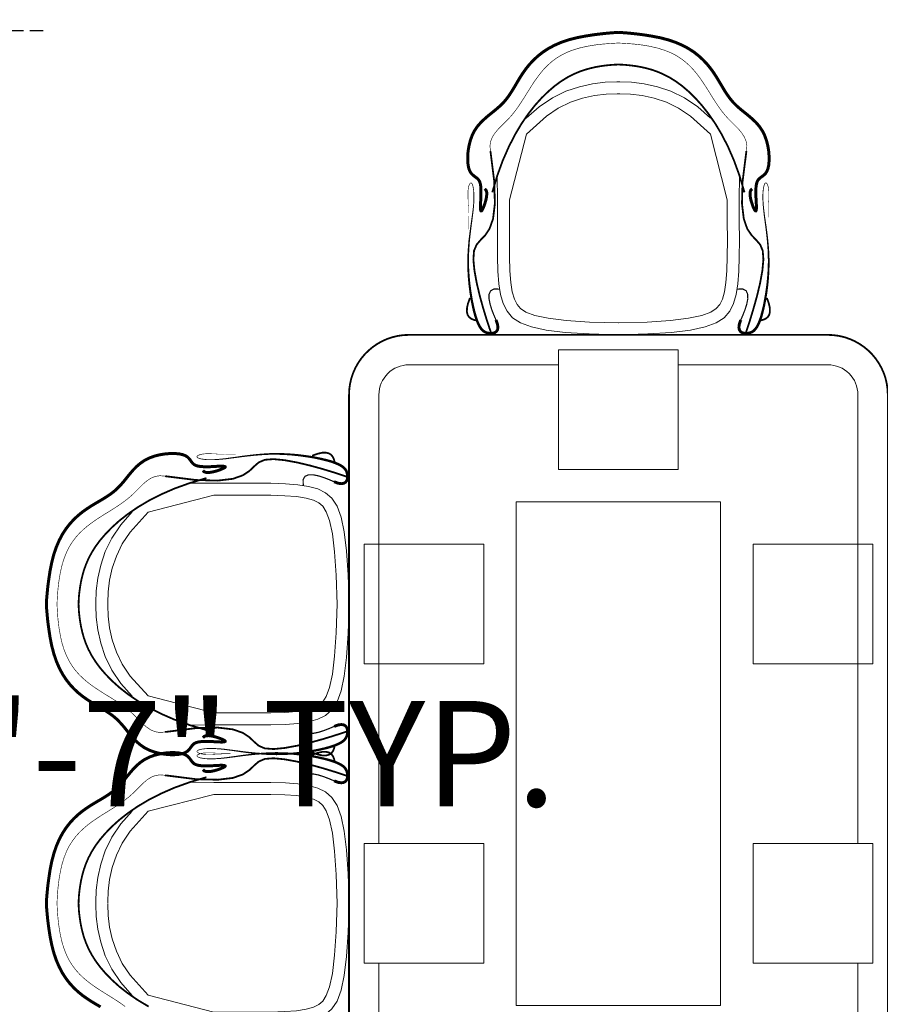
# Model space of a CAD drawing. Units: inches. Extents: x 513 to 1142, y 396 to 927.
# Tile 17 of 31: x 786 to 818, y 728 to 766. Entities that reach past the tile are written whole.
import ezdxf

# ---------------------------------------------------------------- set-up
doc = ezdxf.new("R2010")
doc.units = ezdxf.units.IN
doc.header["$MEASUREMENT"] = 0
doc.linetypes.add('DASHED', pattern=[0.75, 0.5, -0.25])
doc.layers.add('A-ANNO-DIMS', color=2, linetype='DASHED', lineweight=18)
doc.layers.add('furniture', color=92, linetype='Continuous', lineweight=18)
doc.styles.get("Standard").update_dxf_attribs({"font": 'arial.ttf'})
doc.dimstyles.get("Standard").update_dxf_attribs({"dimtxt": 4, "dimasz": 0.18, "dimexe": 0.18, "dimexo": 0.0625, "dimgap": 0.09, "dimtad": 0, "dimtih": 1, "dimtoh": 1, "dimdec": 0, "dimrnd": 6, "dimzin": 0, "dimdsep": 46, "dimlunit": 3, "dimtxsty": 'Standard', "dimcen": 0.09, "dimadec": 0, "dimazin": 0, "dimtfac": 1, "dimtdec": 0, "dimtofl": 0, "dimtmove": 0, "dimatfit": 3, "dimfxl": 1, "dimtolj": 1, "dimtzin": 0, "dimarcsym": 0})

# ---------------------------------------------------------------- blocks, each defined once
blk = doc.blocks.new('ОГ55_на6персон_стол1400х900')
for points, const_width in [([(-423.2, 694.5), (-418.9, 701.9), (-414.4, 709.4), (-409.5, 716.9), (-404.2, 724.4), (-398.3, 731.7), (-391.7, 738.8), (-384.3, 745.6), (-376.1, 752), (-366.9, 758), (-356.7, 763.4), (-345.4, 768.3), (-333, 772.5), (-319.5, 776), (-305.4, 778.8), (-291.5, 780.9), (-278.6, 782.6), (-267.2, 783.7), (-258.2, 784.5), (-252.2, 784.9), (-250, 785)], 5), ([(-26.6, 523.4), (-28.8, 521.4), (-29.9, 518.2), (-30.1, 514.2), (-29.6, 509.6), (-28.6, 504.8), (-27.3, 500.1), (-25.8, 495.7), (-24.3, 492), (-23, 489.2), (-22, 487.3), (-21.1, 486.4), (-20.4, 486.4), (-19.9, 487.3), (-19.6, 489.1), (-19.4, 491.8), (-19.5, 495.4), (-19.7, 499.8), (-20, 504.9), (-20.3, 510.3), (-20.4, 516), (-20.4, 521.5), (-20.1, 526.8), (-19.4, 531.5), (-18.2, 535.5), (-16.5, 538.5), (-14.3, 540.8), (-11.8, 542.8), (-9.2, 544.6), (-6.6, 546.7), (-4.1, 549.3), (-1.9, 552.7), (-0.2, 557.2), (1.1, 563.1), (1.7, 570.2), (1.7, 578.1), (1, 586.6), (-0.4, 595.4), (-2.6, 604.2), (-5.7, 612.7), (-9.6, 620.6), (-14.5, 627.7), (-20, 634.2), (-26.1, 640.1), (-32.5, 645.6), (-39.1, 650.9), (-45.7, 656.2), (-51.9, 661.7), (-57.8, 667.5), (-63.1, 673.7), (-67.9, 680.3), (-72.4, 687.3), (-76.8, 694.5), (-81.1, 701.9), (-85.6, 709.4), (-90.5, 716.9), (-95.8, 724.4), (-101.7, 731.7), (-108.3, 738.8), (-115.7, 745.6), (-123.9, 752), (-133.1, 758), (-143.3, 763.4), (-154.6, 768.3), (-167, 772.5), (-180.5, 776), (-194.6, 778.8), (-208.5, 780.9), (-221.4, 782.6), (-232.8, 783.7), (-241.8, 784.5), (-247.8, 784.9), (-250, 785)], 5), ([(26.6, 523.4), (28.8, 521.4), (29.9, 518.2), (30.1, 514.2), (29.6, 509.6), (28.6, 504.8), (27.3, 500.1), (25.8, 495.7), (24.3, 492), (23, 489.2), (22, 487.3), (21.1, 486.4), (20.4, 486.4), (19.9, 487.3), (19.6, 489.1), (19.4, 491.8), (19.5, 495.4), (19.7, 499.8), (20, 504.9), (20.3, 510.3), (20.4, 516), (20.4, 521.5), (20.1, 526.8), (19.4, 531.5), (18.2, 535.5), (16.5, 538.5), (14.3, 540.8), (11.8, 542.8), (9.2, 544.6), (6.6, 546.7), (4.1, 549.3), (1.9, 552.7), (0.2, 557.2), (-1.1, 563.1), (-1.7, 570.2), (-1.7, 578.1), (-1, 586.6), (0.4, 595.4), (2.6, 604.2), (5.7, 612.7), (9.6, 620.6), (14.5, 627.7), (20, 634.2), (26.1, 640.1), (32.5, 645.6), (39.1, 650.9), (45.7, 656.2), (51.9, 661.7), (57.8, 667.5), (63.1, 673.7), (67.9, 680.3), (72.4, 687.3), (76.8, 694.5), (81.1, 701.9), (85.6, 709.4), (90.5, 716.9), (95.8, 724.4), (101.7, 731.7), (108.3, 738.8), (115.7, 745.6), (123.9, 752), (133.1, 758), (143.3, 763.4), (154.6, 768.3), (167, 772.5), (180.5, 776), (194.6, 778.8), (208.5, 780.9), (221.4, 782.6), (232.8, 783.7), (241.8, 784.5), (247.8, 784.9), (250, 785)], 5), ([(473.4, 523.4), (471.2, 521.4), (470.1, 518.2), (469.9, 514.2), (470.4, 509.6), (471.4, 504.8), (472.7, 500.1), (474.2, 495.7), (475.7, 492), (477, 489.2), (478, 487.3), (478.9, 486.4), (479.6, 486.4), (480.1, 487.3), (480.4, 489.1), (480.6, 491.8), (480.5, 495.4), (480.3, 499.8), (480, 504.9), (479.7, 510.3), (479.6, 516), (479.6, 521.5), (479.9, 526.8), (480.6, 531.5), (481.8, 535.5), (483.5, 538.5), (485.7, 540.8), (488.2, 542.8), (490.8, 544.6), (493.4, 546.7), (495.9, 549.3), (498.1, 552.7), (499.8, 557.2), (501.1, 563.1), (501.7, 570.2), (501.7, 578.1), (501, 586.6), (499.6, 595.4), (497.4, 604.2), (494.3, 612.7), (490.4, 620.6), (485.5, 627.7), (480, 634.2), (473.9, 640.1), (467.5, 645.6), (460.9, 650.9), (454.3, 656.2), (448.1, 661.7), (442.2, 667.5), (436.9, 673.7), (432.1, 680.3), (427.6, 687.3), (423.2, 694.5), (418.9, 701.9), (414.4, 709.4), (409.5, 716.9), (404.2, 724.4), (398.3, 731.7), (391.7, 738.8), (384.3, 745.6), (376.1, 752), (366.9, 758), (356.7, 763.4), (345.4, 768.3), (333, 772.5), (319.5, 776), (305.4, 778.8), (291.5, 780.9), (278.6, 782.6), (267.2, 783.7), (258.2, 784.5), (252.2, 784.9), (250, 785)], 5), ([(-422.8, 653.3), (-417.9, 659.9), (-413.3, 666.7), (-408.8, 673.7), (-404.4, 680.7), (-400, 687.9), (-395.5, 695), (-390.8, 702.2), (-385.8, 709.3), (-380.5, 716.3), (-374.7, 723.1), (-368.5, 729.6), (-361.7, 735.7), (-354.1, 741.4), (-345.9, 746.6), (-336.7, 751.2), (-326.7, 755.2), (-315.5, 758.7), (-303.3, 761.5), (-289.8, 763.8), (-274.9, 765.6), (-258.6, 766.8), (-250, 767.1)], 1), ([(-36.2, 586.5), (-35.4, 595.2), (-36.6, 603), (-39.5, 610.1), (-43.7, 616.6), (-48.9, 622.8), (-54.7, 628.7), (-60.7, 634.6), (-66.6, 640.6), (-72.1, 646.8), (-77.2, 653.3), (-82.1, 659.9), (-86.7, 666.7), (-91.2, 673.7), (-95.6, 680.7), (-100, 687.9), (-104.5, 695), (-109.2, 702.2), (-114.2, 709.3), (-119.5, 716.3), (-125.3, 723.1), (-131.5, 729.6), (-138.3, 735.7), (-145.9, 741.4), (-154.1, 746.6), (-163.3, 751.2), (-173.3, 755.2), (-184.5, 758.7), (-196.7, 761.5), (-210.2, 763.8), (-225.1, 765.6), (-241.4, 766.8), (-250, 767.1)], 1), ([(36.2, 586.5), (35.4, 595.2), (36.6, 603), (39.5, 610.1), (43.7, 616.6), (48.9, 622.8), (54.7, 628.7), (60.7, 634.6), (66.6, 640.6), (72.1, 646.8), (77.2, 653.3), (82.1, 659.9), (86.7, 666.7), (91.2, 673.7), (95.6, 680.7), (100, 687.9), (104.5, 695), (109.2, 702.2), (114.2, 709.3), (119.5, 716.3), (125.3, 723.1), (131.5, 729.6), (138.3, 735.7), (145.9, 741.4), (154.1, 746.6), (163.3, 751.2), (173.3, 755.2), (184.5, 758.7), (196.7, 761.5), (210.2, 763.8), (225.1, 765.6), (241.4, 766.8), (250, 767.1)], 1), ([(463.8, 586.5), (464.6, 595.2), (463.4, 603), (460.5, 610.1), (456.3, 616.6), (451.1, 622.8), (445.3, 628.7), (439.3, 634.6), (433.4, 640.6), (427.9, 646.8), (422.8, 653.3), (417.9, 659.9), (413.3, 666.7), (408.8, 673.7), (404.4, 680.7), (400, 687.9), (395.5, 695), (390.8, 702.2), (385.8, 709.3), (380.5, 716.3), (374.7, 723.1), (368.5, 729.6), (361.7, 735.7), (354.1, 741.4), (345.9, 746.6), (336.7, 751.2), (326.7, 755.2), (315.5, 758.7), (303.3, 761.5), (289.8, 763.8), (274.9, 765.6), (258.6, 766.8), (250, 767.1)], 1), ([(-422.7, 614.1), (-411.8, 632.4), (-400.6, 648.7), (-389.4, 663), (-378.2, 675.4), (-367.2, 686.1), (-356.5, 695.3), (-346, 703), (-335.8, 709.4), (-325.7, 714.7), (-315.9, 718.9), (-306.4, 722.3), (-297, 724.9), (-287.9, 727), (-279.3, 728.5), (-271.3, 729.6), (-264.3, 730.4), (-258.4, 730.8), (-253.9, 731), (-251, 731.1), (-250, 731.1)], 3), ([(-39.4, 517.6), (-47.7, 545.4), (-56.8, 570.7), (-66.8, 593.6), (-77.3, 614.1), (-88.2, 632.4), (-99.4, 648.7), (-110.6, 663), (-121.8, 675.4), (-132.8, 686.1), (-143.5, 695.3), (-154, 703), (-164.2, 709.4), (-174.3, 714.7), (-184.1, 718.9), (-193.6, 722.3), (-203, 724.9), (-212.1, 727), (-220.7, 728.5), (-228.7, 729.6), (-235.7, 730.4), (-241.6, 730.8), (-246.1, 731), (-249, 731.1), (-250, 731.1)], 3), ([(39.4, 517.6), (47.7, 545.4), (56.8, 570.7), (66.8, 593.6), (77.3, 614.1), (88.2, 632.4), (99.4, 648.7), (110.6, 663), (121.8, 675.4), (132.8, 686.1), (143.5, 695.3), (154, 703), (164.2, 709.4), (174.3, 714.7), (184.1, 718.9), (193.6, 722.3), (203, 724.9), (212.1, 727), (220.7, 728.5), (228.7, 729.6), (235.7, 730.4), (241.6, 730.8), (246.1, 731), (249, 731.1), (250, 731.1)], 3), ([(460.6, 517.6), (452.3, 545.4), (443.2, 570.7), (433.2, 593.6), (422.7, 614.1), (411.8, 632.4), (400.6, 648.7), (389.4, 663), (378.2, 675.4), (367.2, 686.1), (356.5, 695.3), (346, 703), (335.8, 709.4), (325.7, 714.7), (315.9, 718.9), (306.4, 722.3), (297, 724.9), (287.9, 727), (279.3, 728.5), (271.3, 729.6), (264.3, 730.4), (258.4, 730.8), (253.9, 731), (251, 731.1), (250, 731.1)], 3), ([(-36.2, 586.5), (-42.6, 535.5), (-43.6, 498.8), (-40.6, 473.4), (-34.7, 456.6), (-27.4, 445.7), (-19.8, 437.8), (-13.2, 430.2), (-8.8, 420), (-7.7, 405.3), (-9.5, 386.7), (-13.3, 366), (-18.4, 344.5), (-24.1, 323.8), (-29.7, 305.4), (-34.4, 291), (-37.5, 281.9)], 3), ([(36.2, 586.5), (42.6, 535.5), (43.6, 498.8), (40.6, 473.4), (34.7, 456.6), (27.4, 445.7), (19.8, 437.8), (13.2, 430.2), (8.8, 420), (7.7, 405.3), (9.5, 386.7), (13.3, 366), (18.4, 344.5), (24.1, 323.8), (29.7, 305.4), (34.4, 291), (37.5, 281.9)], 3), ([(463.8, 586.5), (457.4, 535.5), (456.4, 498.8), (459.4, 473.4), (465.3, 456.6), (472.6, 445.7), (480.2, 437.8), (486.8, 430.2), (491.2, 420), (492.3, 405.3), (490.5, 386.7), (486.7, 366), (481.6, 344.5), (475.9, 323.8), (470.3, 305.4), (465.6, 291), (462.5, 281.9)], 3), ([(-45.5, 304.2), (-42.2, 312), (-38.7, 321), (-35.7, 330.3), (-33.9, 339.3), (-34, 347.1), (-36.5, 353), (-42.2, 356.1), (-51.8, 355.7)], 2), ([(45.5, 304.2), (42.2, 312), (38.7, 321), (35.7, 330.3), (33.9, 339.3), (34, 347.1), (36.5, 353), (42.2, 356.1), (51.8, 355.7)], 2), ([(454.5, 304.2), (457.8, 312), (461.3, 321), (464.3, 330.3), (466.1, 339.3), (466, 347.1), (463.5, 353), (457.8, 356.1), (448.2, 355.7)], 2), ([(-2, 341), (1.3, 331.8), (3, 324.1), (3.1, 317.8), (1.9, 312.9), (-0.6, 309), (-4.2, 306.2), (-8.8, 304.3), (-14.3, 303.1)], 3), ([(2, 341), (-1.3, 331.8), (-3, 324.1), (-3.1, 317.8), (-1.9, 312.9), (0.6, 309), (4.2, 306.2), (8.8, 304.3), (14.3, 303.1)], 3), ([(498, 341), (501.3, 331.8), (503, 324.1), (503.1, 317.8), (501.9, 312.9), (499.4, 309), (495.8, 306.2), (491.2, 304.3), (485.7, 303.1)], 3), ([(761.7, 77.3), (752.5, 80.6), (744.8, 82.3), (738.5, 82.4), (733.5, 81.2), (729.7, 78.7), (726.9, 75.1), (725, 70.5), (723.8, 65)], 3), ([(944.1, 52.8), (942.1, 50.6), (938.9, 49.4), (934.9, 49.2), (930.3, 49.7), (925.5, 50.7), (920.8, 52), (916.4, 53.5), (912.7, 55), (909.9, 56.3), (908, 57.4), (907.1, 58.2), (907.1, 58.9), (908, 59.4), (909.8, 59.7), (912.5, 59.9), (916.1, 59.8), (920.5, 59.6), (925.5, 59.3), (931, 59), (936.6, 58.9), (942.2, 58.9), (947.5, 59.2), (952.2, 59.9), (956.2, 61.1), (959.2, 62.9), (961.5, 65), (963.4, 67.5), (965.3, 70.1), (967.4, 72.7), (969.9, 75.2), (973.4, 77.4), (977.9, 79.2), (983.8, 80.4), (990.9, 81.1), (998.8, 81.1), (1007.3, 80.4), (1016.1, 78.9), (1024.9, 76.7), (1033.4, 73.6), (1041.3, 69.7), (1048.4, 64.9), (1054.8, 59.3), (1060.7, 53.2), (1066.3, 46.8), (1071.6, 40.2), (1076.9, 33.7), (1082.4, 27.4), (1088.1, 21.5), (1094.4, 16.2), (1101, 11.4), (1108, 6.9), (1115.2, 2.5), (1122.6, -1.8), (1130.1, -6.3), (1137.6, -11.1), (1145, -16.4), (1152.3, -22.3), (1159.4, -29), (1166.2, -36.3), (1172.7, -44.6), (1178.7, -53.8), (1184.1, -64), (1189, -75.2), (1193.2, -87.7), (1196.7, -101.2), (1199.4, -115.3), (1201.6, -129.2), (1203.2, -142.1), (1204.4, -153.5), (1205.1, -162.5), (1205.5, -168.5), (1205.7, -170.7)], 5), ([(1007.2, 43.1), (956.2, 36.7), (919.4, 35.7), (894.1, 38.7), (877.3, 44.6), (866.4, 51.9), (858.5, 59.6), (850.8, 66.2), (840.7, 70.5), (826, 71.6), (807.4, 69.8), (786.6, 66), (765.2, 60.9), (744.5, 55.2), (726.1, 49.6), (711.6, 44.9), (702.6, 41.8)], 3), ([(724.9, 33.8), (732.7, 37.2), (741.6, 40.7), (751, 43.6), (760, 45.4), (767.8, 45.4), (773.6, 42.8), (776.8, 37.1), (776.4, 27.6)], 2), ([(938.3, 40), (966.1, 31.7), (991.4, 22.5), (1014.2, 12.5), (1034.8, 2), (1053.1, -8.9), (1069.4, -20.1), (1083.7, -31.3), (1096.1, -42.5), (1106.8, -53.5), (1116, -64.2), (1123.7, -74.7), (1130.1, -84.9), (1135.3, -94.9), (1139.6, -104.7), (1143, -114.3), (1145.6, -123.7), (1147.7, -132.7), (1149.2, -141.4), (1150.3, -149.3), (1151, -156.4), (1151.5, -162.3), (1151.7, -166.8), (1151.8, -169.6), (1151.8, -170.7)], 3), ([(1007.2, 43.1), (1015.9, 43.9), (1023.6, 42.7), (1030.7, 39.8), (1037.3, 35.6), (1043.5, 30.4), (1049.4, 24.7), (1055.3, 18.6), (1061.3, 12.7), (1067.5, 7.2), (1073.9, 2.1), (1080.6, -2.8), (1087.4, -7.4), (1094.3, -11.8), (1101.4, -16.3), (1108.5, -20.7), (1115.7, -25.2), (1122.9, -29.9), (1130, -34.9), (1137, -40.2), (1143.8, -45.9), (1150.3, -52.2), (1156.4, -59), (1162.1, -66.5), (1167.3, -74.8), (1171.9, -83.9), (1175.9, -94), (1179.3, -105.1), (1182.2, -117.4), (1184.5, -130.9), (1186.2, -145.8), (1187.4, -162.1), (1187.8, -170.7)], 1), ([(944.1, -394.1), (942.1, -391.9), (938.9, -390.8), (934.9, -390.6), (930.3, -391.1), (925.5, -392), (920.8, -393.4), (916.4, -394.9), (912.7, -396.3), (909.9, -397.6), (908, -398.7), (907.1, -399.6), (907.1, -400.3), (908, -400.8), (909.8, -401.1), (912.5, -401.2), (916.1, -401.2), (920.5, -401), (925.5, -400.7), (931, -400.4), (936.6, -400.2), (942.2, -400.3), (947.5, -400.6), (952.2, -401.3), (956.2, -402.5), (959.2, -404.2), (961.5, -406.4), (963.4, -408.8), (965.3, -411.4), (967.4, -414.1), (969.9, -416.5), (973.4, -418.7), (977.9, -420.5), (983.8, -421.8), (990.9, -422.4), (998.8, -422.4), (1007.3, -421.7), (1016.1, -420.3), (1024.9, -418), (1033.4, -415), (1041.3, -411), (1048.4, -406.2), (1054.8, -400.7), (1060.7, -394.6), (1066.3, -388.1), (1071.6, -381.6), (1076.9, -375), (1082.4, -368.7), (1088.1, -362.9), (1094.4, -357.6), (1101, -352.8), (1108, -348.2), (1115.2, -343.9), (1122.6, -339.5), (1130.1, -335), (1137.6, -330.2), (1145, -324.9), (1152.3, -319), (1159.4, -312.4), (1166.2, -305), (1172.7, -296.8), (1178.7, -287.6), (1184.1, -277.4), (1189, -266.1), (1193.2, -253.7), (1196.7, -240.1), (1199.4, -226.1), (1201.6, -212.2), (1203.2, -199.2), (1204.4, -187.9), (1205.1, -178.9), (1205.5, -172.9), (1205.7, -170.7)], 5), ([(938.3, -381.3), (966.1, -373), (991.4, -363.8), (1014.2, -353.9), (1034.8, -343.4), (1053.1, -332.5), (1069.4, -321.3), (1083.7, -310), (1096.1, -298.9), (1106.8, -287.9), (1116, -277.2), (1123.7, -266.7), (1130.1, -256.4), (1135.3, -246.4), (1139.6, -236.6), (1143, -227), (1145.6, -217.7), (1147.7, -208.6), (1149.2, -200), (1150.3, -192), (1151, -185), (1151.5, -179.1), (1151.7, -174.6), (1151.8, -171.7), (1151.8, -170.7)], 3), ([(1007.2, -384.5), (1015.9, -385.3), (1023.6, -384), (1030.7, -381.1), (1037.3, -376.9), (1043.5, -371.8), (1049.4, -366), (1055.3, -360), (1061.3, -354.1), (1067.5, -348.6), (1073.9, -343.4), (1080.6, -338.6), (1087.4, -334), (1094.3, -329.5), (1101.4, -325.1), (1108.5, -320.7), (1115.7, -316.1), (1122.9, -311.4), (1130, -306.5), (1137, -301.2), (1143.8, -295.4), (1150.3, -289.2), (1156.4, -282.3), (1162.1, -274.8), (1167.3, -266.5), (1171.9, -257.4), (1175.9, -247.3), (1179.3, -236.2), (1182.2, -224), (1184.5, -210.5), (1186.2, -195.6), (1187.4, -179.3), (1187.8, -170.7)], 1), ([(1007.2, -384.5), (956.2, -378.1), (919.4, -377.1), (894.1, -380.1), (877.3, -385.9), (866.4, -393.3), (858.5, -400.9), (850.8, -407.5), (840.7, -411.8), (826, -412.9), (807.4, -411.2), (786.6, -407.4), (765.2, -402.3), (744.5, -396.5), (726.1, -391), (711.6, -386.3), (702.6, -383.2)], 3), ([(724.9, -375.1), (732.7, -378.5), (741.6, -382), (751, -385), (760, -386.8), (767.8, -386.7), (773.6, -384.2), (776.8, -378.4), (776.4, -368.9)], 2), ([(761.7, -418.7), (752.5, -422), (744.8, -423.7), (738.5, -423.8), (733.5, -422.6), (729.7, -420.1), (726.9, -416.5), (725, -411.9), (723.8, -406.4)], 3)]:
    blk.add_lwpolyline(points, dxfattribs=dict(const_width=const_width))
for points in [[(-404, 641.6), (-382.6, 660.8), (-360.4, 675.6), (-337.8, 686.5), (-315.2, 694.2), (-293.1, 699), (-272, 701.6), (-252.3, 702.5), (-250, 702.4)], [(-96, 641.6), (-117.4, 660.8), (-139.6, 675.6), (-162.2, 686.5), (-184.8, 694.2), (-206.9, 699), (-228, 701.6), (-247.7, 702.5), (-250, 702.4)], [(96, 641.6), (117.4, 660.8), (139.6, 675.6), (162.2, 686.5), (184.8, 694.2), (206.9, 699), (228, 701.6), (247.7, 702.5), (250, 702.4)], [(404, 641.6), (382.6, 660.8), (360.4, 675.6), (337.8, 686.5), (315.2, 694.2), (293.1, 699), (272, 701.6), (252.3, 702.5), (250, 702.4)], [(-403.6, 615), (-370.3, 644.9), (-350.5, 658.2), (-330.2, 668), (-309.8, 674.9), (-289.8, 679.3), (-270.4, 681.7), (-252.1, 682.5), (-250.4, 682.4)], [(-96.4, 615), (-129.7, 644.9), (-149.5, 658.2), (-169.8, 668), (-190.2, 674.9), (-210.2, 679.3), (-229.6, 681.7), (-247.9, 682.5), (-249.6, 682.4)], [(96.4, 615), (129.7, 644.9), (149.5, 658.2), (169.8, 668), (190.2, 674.9), (210.2, 679.3), (229.6, 681.7), (247.9, 682.5), (249.6, 682.4)], [(403.6, 615), (370.3, 644.9), (350.5, 658.2), (330.2, 668), (309.8, 674.9), (289.8, 679.3), (270.4, 681.7), (252.1, 682.5), (250.4, 682.4)], [(-403.6, 615), (-431.9, 505.2), (-431.9, 469.2), (-432, 437.6), (-431.9, 410.1), (-431.2, 386.6), (-429.8, 367), (-427.3, 351.1), (-423.8, 338.8), (-419.4, 329.9), (-413.6, 323.3), (-404.4, 317.4), (-389.5, 311.8), (-367.3, 307), (-337.1, 303.4), (-298.1, 300.9), (-249.4, 299.3)], [(-96.4, 615), (-68.1, 505.2), (-68.1, 469.2), (-68, 437.6), (-68.1, 410.1), (-68.8, 386.6), (-70.2, 367), (-72.7, 351.1), (-76.2, 338.8), (-80.6, 329.9), (-86.4, 323.3), (-95.6, 317.4), (-110.5, 311.8), (-132.7, 307), (-162.9, 303.4), (-201.9, 300.9), (-250.6, 299.3)], [(96.4, 615), (68.1, 505.2), (68.1, 469.2), (68, 437.6), (68.1, 410.1), (68.8, 386.6), (70.2, 367), (72.7, 351.1), (76.2, 338.8), (80.6, 329.9), (86.4, 323.3), (95.6, 317.4), (110.5, 311.8), (132.7, 307), (162.9, 303.4), (201.9, 300.9), (250.6, 299.3)], [(403.6, 615), (431.9, 505.2), (431.9, 469.2), (432, 437.6), (431.9, 410.1), (431.2, 386.6), (429.8, 367), (427.3, 351.1), (423.8, 338.8), (419.4, 329.9), (413.6, 323.3), (404.4, 317.4), (389.5, 311.8), (367.3, 307), (337.1, 303.4), (298.1, 300.9), (249.4, 299.3)], [(-452.3, 545.4), (-451.9, 505.1), (-451.9, 469.2), (-452, 437.5), (-451.9, 409.8), (-451.2, 385.6), (-449.6, 364.7), (-446.8, 346.8), (-442.5, 331.5), (-436.1, 318.7), (-426.8, 308), (-413.5, 299.4), (-395.1, 292.5), (-370.6, 287.3), (-339, 283.5), (-299.1, 280.9), (-250, 279.3)], [(-47.7, 545.4), (-48.1, 505.1), (-48.1, 469.2), (-48, 437.5), (-48.1, 409.8), (-48.8, 385.6), (-50.4, 364.7), (-53.2, 346.8), (-57.5, 331.5), (-63.9, 318.7), (-73.2, 308), (-86.5, 299.4), (-104.9, 292.5), (-129.4, 287.3), (-161, 283.5), (-200.9, 280.9), (-250, 279.3)], [(47.7, 545.4), (48.1, 505.1), (48.1, 469.2), (48, 437.5), (48.1, 409.8), (48.8, 385.6), (50.4, 364.7), (53.2, 346.8), (57.5, 331.5), (63.9, 318.7), (73.2, 308), (86.5, 299.4), (104.9, 292.5), (129.4, 287.3), (161, 283.5), (200.9, 280.9), (250, 279.3)], [(452.3, 545.4), (451.9, 505.1), (451.9, 469.2), (452, 437.5), (451.9, 409.8), (451.2, 385.6), (449.6, 364.7), (446.8, 346.8), (442.5, 331.5), (436.1, 318.7), (426.8, 308), (413.5, 299.4), (395.1, 292.5), (370.6, 287.3), (339, 283.5), (299.1, 280.9), (250, 279.3)], [(966.1, 31.7), (925.8, 31.2), (889.9, 31.2), (858.2, 31.3), (830.4, 31.2), (806.3, 30.5), (785.4, 29), (767.4, 26.2), (752.2, 21.8), (739.4, 15.4), (728.7, 6.1), (720.1, -7.2), (713.2, -25.6), (708, -50.1), (704.2, -81.7), (701.6, -121.6), (700, -170.7)], [(1035.7, -17.1), (925.9, 11.2), (889.9, 11.2), (858.2, 11.3), (830.8, 11.2), (807.3, 10.5), (787.6, 9.1), (771.7, 6.6), (759.5, 3.1), (750.6, -1.3), (744, -7.1), (738, -16.3), (732.5, -31.2), (727.7, -53.4), (724.1, -83.6), (721.5, -122.5), (720, -171.3)], [(1035.7, -17.1), (1065.6, -50.4), (1078.8, -70.2), (1088.7, -90.5), (1095.5, -110.8), (1100, -130.9), (1102.3, -150.3), (1103.1, -168.6), (1103.1, -170.3)], [(1062.3, -16.7), (1081.4, -38.1), (1096.2, -60.3), (1107.2, -82.9), (1114.8, -105.5), (1119.7, -127.5), (1122.3, -148.6), (1123.1, -168.3), (1123.1, -170.7)], [(966.1, -373), (925.8, -372.6), (889.9, -372.6), (858.2, -372.7), (830.4, -372.6), (806.3, -371.9), (785.4, -370.3), (767.4, -367.5), (752.2, -363.2), (739.4, -356.8), (728.7, -347.5), (720.1, -334.1), (713.2, -315.8), (708, -291.3), (704.2, -259.6), (701.6, -219.8), (700, -170.7)], [(1035.7, -324.3), (925.9, -352.6), (889.9, -352.6), (858.2, -352.7), (830.8, -352.6), (807.3, -351.9), (787.6, -350.4), (771.7, -348), (759.5, -344.4), (750.6, -340), (744, -334.2), (738, -325.1), (732.5, -310.2), (727.7, -288), (724.1, -257.8), (721.5, -218.8), (720, -170)], [(1035.7, -324.3), (1065.6, -291), (1078.8, -271.1), (1088.7, -250.9), (1095.5, -230.5), (1100, -210.5), (1102.3, -191.1), (1103.1, -172.8), (1103.1, -171.1)], [(1062.3, -324.6), (1081.4, -303.3), (1096.2, -281.1), (1107.2, -258.5), (1114.8, -235.9), (1119.7, -213.8), (1122.3, -192.7), (1123.1, -173), (1123.1, -170.7)]]:
    blk.add_lwpolyline(points)
for points, format in [([(-45.5, 304.2, 5, 4.91, 0), (-48, 297.4, 4.91, 4.84, 0), (-48.7, 292.1, 4.84, 4.78, 0), (-48.1, 288.1, 4.78, 4.74, 0), (-46.3, 285.1, 4.74, 4.7, 0), (-43.7, 283.2, 4.7, 4.65, 0), (-40.6, 282.2, 4.65, 4.61, 0), (-37.1, 281.8, 4.61, 4.56, 0), (-33.5, 282.1, 4.56, 4.52, 0), (-30.2, 282.8, 4.52, 4.47, 0), (-27.1, 284.1, 4.47, 4.43, 0), (-24.1, 286.1, 4.43, 4.38, 0), (-21.3, 288.8, 4.38, 4.32, 0), (-18.7, 292.5, 4.32, 4.25, 0), (-16.2, 297.3, 4.25, 4.17, 0), (-13.7, 303.2, 4.17, 4.07, 0), (-11.3, 310.4, 4.07, 3.95, 0), (-9, 318.9, 3.95, 3.82, 0), (-6.7, 328.7, 3.82, 3.68, 0), (-4.6, 339.4, 3.68, 3.53, 0), (-2.8, 350.9, 3.53, 3.37, 0), (-1.2, 363, 3.37, 3.21, 0), (0, 375.5, 3.21, 3.05, 0), (0.8, 388.2, 3.05, 2.88, 0), (1.1, 400.7, 2.88, 2.72, 0), (0.9, 413.1, 2.72, 2.57, 0), (0.2, 425.1, 2.57, 2.41, 0), (-0.8, 436.7, 2.41, 2.27, 0), (-2, 447.8, 2.27, 2.13, 0), (-3.3, 458.3, 2.13, 2, 0), (-4.7, 468.2, 2, 1.88, 0), (-5.9, 477.3, 1.88, 1.78, 0), (-7, 485.6, 1.78, 1.68, 0), (-7.8, 493.1, 1.68, 1.59, 0), (-8.3, 499.6, 1.59, 1.52, 0), (-8.6, 505.4, 1.52, 1.45, 0), (-8.7, 510.5, 1.45, 1.4, 0), (-8.6, 514.9, 1.4, 1.35, 0), (-8.4, 518.7, 1.35, 1.3, 0), (-8, 521.9, 1.3, 1.27, 0), (-7.6, 524.7, 1.27, 1.24, 0), (-7.2, 527, 1.24, 1.21, 0), (-6.7, 528.8, 1.21, 1.19, 0), (-6.2, 530.3, 1.19, 1.18, 0), (-5.7, 531.5, 1.18, 1.16, 0), (-5.2, 532.3, 1.16, 1.15, 0), (-4.7, 532.9, 1.15, 1.14, 0), (-4.2, 533.2, 1.14, 1.14, 0), (-3.7, 533.3, 1.14, 1.13, 0), (-3.2, 533.2, 1.13, 1.12, 0), (-2.7, 533, 1.12, 1.12, 0), (-2.2, 532.5, 1.12, 1.11, 0), (-1.7, 531.9, 1.11, 1.09, 0), (-1.3, 531.1, 1.09, 1.08, 0), (-0.9, 530.2, 1.08, 1.07, 0), (-0.5, 529.1, 1.07, 1.05, 0), (-0.1, 527.9, 1.05, 1.03, 0), (0.3, 526.5, 1.03, 1.01, 0), (0.6, 524.9, 1.01, 0.986, 0), (0.9, 523.1, 0.986, 0.959, 0), (1.1, 521, 0.959, 0.926, 0), (1.3, 518.5, 0.926, 0.889, 0), (1.4, 515.7, 0.889, 0.846, 0), (1.4, 512.3, 0.846, 0.796, 0), (1.3, 508.5, 0.796, 0.738, 0), (1.1, 504, 0.738, 0.672, 0), (0.8, 498.9, 0.672, 0.595, 0), (0.6, 493, 0.595, 0.506, 0), (0.3, 486.1, 0.506, 0.404, 0), (0.1, 478.2, 0.404, 0.286, 0), (-0.1, 469.2, 0.286, 0.152, 0), (-0.1, 458.8, 0.152, 0, 0), (0, 447.1, 0, 0, 0)], "xyseb"), ([(45.5, 304.2, 5, 4.91, 0), (48, 297.4, 4.91, 4.84, 0), (48.7, 292.1, 4.84, 4.78, 0), (48.1, 288.1, 4.78, 4.74, 0), (46.3, 285.1, 4.74, 4.7, 0), (43.7, 283.2, 4.7, 4.65, 0), (40.6, 282.2, 4.65, 4.61, 0), (37.1, 281.8, 4.61, 4.56, 0), (33.5, 282.1, 4.56, 4.52, 0), (30.2, 282.8, 4.52, 4.47, 0), (27.1, 284.1, 4.47, 4.43, 0), (24.1, 286.1, 4.43, 4.38, 0), (21.3, 288.8, 4.38, 4.32, 0), (18.7, 292.5, 4.32, 4.25, 0), (16.2, 297.3, 4.25, 4.17, 0), (13.7, 303.2, 4.17, 4.07, 0), (11.3, 310.4, 4.07, 3.95, 0), (9, 318.9, 3.95, 3.82, 0), (6.7, 328.7, 3.82, 3.68, 0), (4.6, 339.4, 3.68, 3.53, 0), (2.8, 350.9, 3.53, 3.37, 0), (1.2, 363, 3.37, 3.21, 0), (0, 375.5, 3.21, 3.05, 0), (-0.8, 388.2, 3.05, 2.88, 0), (-1.1, 400.7, 2.88, 2.72, 0), (-0.9, 413.1, 2.72, 2.57, 0), (-0.2, 425.1, 2.57, 2.41, 0), (0.8, 436.7, 2.41, 2.27, 0), (2, 447.8, 2.27, 2.13, 0), (3.3, 458.3, 2.13, 2, 0), (4.7, 468.2, 2, 1.88, 0), (5.9, 477.3, 1.88, 1.78, 0), (7, 485.6, 1.78, 1.68, 0), (7.8, 493.1, 1.68, 1.59, 0), (8.3, 499.6, 1.59, 1.52, 0), (8.6, 505.4, 1.52, 1.45, 0), (8.7, 510.5, 1.45, 1.4, 0), (8.6, 514.9, 1.4, 1.35, 0), (8.4, 518.7, 1.35, 1.3, 0), (8, 521.9, 1.3, 1.27, 0), (7.6, 524.7, 1.27, 1.24, 0), (7.2, 527, 1.24, 1.21, 0), (6.7, 528.8, 1.21, 1.19, 0), (6.2, 530.3, 1.19, 1.18, 0), (5.7, 531.5, 1.18, 1.16, 0), (5.2, 532.3, 1.16, 1.15, 0), (4.7, 532.9, 1.15, 1.14, 0), (4.2, 533.2, 1.14, 1.14, 0), (3.7, 533.3, 1.14, 1.13, 0), (3.2, 533.2, 1.13, 1.12, 0), (2.7, 533, 1.12, 1.12, 0), (2.2, 532.5, 1.12, 1.11, 0), (1.7, 531.9, 1.11, 1.09, 0), (1.3, 531.1, 1.09, 1.08, 0), (0.9, 530.2, 1.08, 1.07, 0), (0.5, 529.1, 1.07, 1.05, 0), (0.1, 527.9, 1.05, 1.03, 0), (-0.3, 526.5, 1.03, 1.01, 0), (-0.6, 524.9, 1.01, 0.986, 0), (-0.9, 523.1, 0.986, 0.959, 0), (-1.1, 521, 0.959, 0.926, 0), (-1.3, 518.5, 0.926, 0.889, 0), (-1.4, 515.7, 0.889, 0.846, 0), (-1.4, 512.3, 0.846, 0.796, 0), (-1.3, 508.5, 0.796, 0.738, 0), (-1.1, 504, 0.738, 0.672, 0), (-0.8, 498.9, 0.672, 0.595, 0), (-0.6, 493, 0.595, 0.506, 0), (-0.3, 486.1, 0.506, 0.404, 0), (-0.1, 478.2, 0.404, 0.286, 0), (0.1, 469.2, 0.286, 0.152, 0), (0.1, 458.8, 0.152, 0, 0), (0, 447.1, 0, 0, 0)], "xyseb"), ([(454.5, 304.2, 5, 4.91, 0), (452, 297.4, 4.91, 4.84, 0), (451.3, 292.1, 4.84, 4.78, 0), (451.9, 288.1, 4.78, 4.74, 0), (453.7, 285.1, 4.74, 4.7, 0), (456.3, 283.2, 4.7, 4.65, 0), (459.4, 282.2, 4.65, 4.61, 0), (462.9, 281.8, 4.61, 4.56, 0), (466.5, 282.1, 4.56, 4.52, 0), (469.8, 282.8, 4.52, 4.47, 0), (472.9, 284.1, 4.47, 4.43, 0), (475.9, 286.1, 4.43, 4.38, 0), (478.7, 288.8, 4.38, 4.32, 0), (481.3, 292.5, 4.32, 4.25, 0), (483.8, 297.3, 4.25, 4.17, 0), (486.3, 303.2, 4.17, 4.07, 0), (488.7, 310.4, 4.07, 3.95, 0), (491, 318.9, 3.95, 3.82, 0), (493.3, 328.7, 3.82, 3.68, 0), (495.4, 339.4, 3.68, 3.53, 0), (497.2, 350.9, 3.53, 3.37, 0), (498.8, 363, 3.37, 3.21, 0), (500, 375.5, 3.21, 3.05, 0), (500.8, 388.2, 3.05, 2.88, 0), (501.1, 400.7, 2.88, 2.72, 0), (500.9, 413.1, 2.72, 2.57, 0), (500.2, 425.1, 2.57, 2.41, 0), (499.2, 436.7, 2.41, 2.27, 0), (498, 447.8, 2.27, 2.13, 0), (496.7, 458.3, 2.13, 2, 0), (495.3, 468.2, 2, 1.88, 0), (494.1, 477.3, 1.88, 1.78, 0), (493, 485.6, 1.78, 1.68, 0), (492.2, 493.1, 1.68, 1.59, 0), (491.7, 499.6, 1.59, 1.52, 0), (491.4, 505.4, 1.52, 1.45, 0), (491.3, 510.5, 1.45, 1.4, 0), (491.4, 514.9, 1.4, 1.35, 0), (491.6, 518.7, 1.35, 1.3, 0), (492, 521.9, 1.3, 1.27, 0), (492.4, 524.7, 1.27, 1.24, 0), (492.8, 527, 1.24, 1.21, 0), (493.3, 528.8, 1.21, 1.19, 0), (493.8, 530.3, 1.19, 1.18, 0), (494.3, 531.5, 1.18, 1.16, 0), (494.8, 532.3, 1.16, 1.15, 0), (495.3, 532.9, 1.15, 1.14, 0), (495.8, 533.2, 1.14, 1.14, 0), (496.3, 533.3, 1.14, 1.13, 0), (496.8, 533.2, 1.13, 1.12, 0), (497.3, 533, 1.12, 1.12, 0), (497.8, 532.5, 1.12, 1.11, 0), (498.3, 531.9, 1.11, 1.09, 0), (498.7, 531.1, 1.09, 1.08, 0), (499.1, 530.2, 1.08, 1.07, 0), (499.5, 529.1, 1.07, 1.05, 0), (499.9, 527.9, 1.05, 1.03, 0), (500.3, 526.5, 1.03, 1.01, 0), (500.6, 524.9, 1.01, 0.986, 0), (500.9, 523.1, 0.986, 0.959, 0), (501.1, 521, 0.959, 0.926, 0), (501.3, 518.5, 0.926, 0.889, 0), (501.4, 515.7, 0.889, 0.846, 0), (501.4, 512.3, 0.846, 0.796, 0), (501.3, 508.5, 0.796, 0.738, 0), (501.1, 504, 0.738, 0.672, 0), (500.8, 498.9, 0.672, 0.595, 0), (500.6, 493, 0.595, 0.506, 0), (500.3, 486.1, 0.506, 0.404, 0), (500.1, 478.2, 0.404, 0.286, 0), (499.9, 469.2, 0.286, 0.152, 0), (499.9, 458.8, 0.152, 0, 0), (500, 447.1, 0, 0, 0)], "xyseb"), ([(-650, -70.7), (-650, 179.3, -0.414214), (-600, 229.3), (-350, 229.3)], "xyb"), ([(-150, 229.3), (600, 229.3, -0.414214), (650, 179.3), (650, -70.7)], "xyb"), ([(724.9, 33.8, 5, 4.91, 0), (718.1, 31.4, 4.91, 4.84, 0), (712.8, 30.6, 4.84, 4.78, 0), (708.7, 31.2, 4.78, 4.74, 0), (705.8, 33, 4.74, 4.7, 0), (703.9, 35.6, 4.7, 4.65, 0), (702.9, 38.8, 4.65, 4.61, 0), (702.5, 42.3, 4.61, 4.56, 0), (702.8, 45.8, 4.56, 4.52, 0), (703.5, 49.1, 4.52, 4.47, 0), (704.8, 52.2, 4.47, 4.43, 0), (706.7, 55.2, 4.43, 4.38, 0), (709.5, 58, 4.38, 4.32, 0), (713.2, 60.6, 4.32, 4.25, 0), (717.9, 63.2, 4.25, 4.17, 0), (723.8, 65.6, 4.17, 4.07, 0), (731, 68, 4.07, 3.95, 0), (739.6, 70.4, 3.95, 3.82, 0), (749.3, 72.6, 3.82, 3.68, 0), (760.1, 74.7, 3.68, 3.53, 0), (771.6, 76.5, 3.53, 3.37, 0), (783.7, 78.1, 3.37, 3.21, 0), (796.2, 79.3, 3.21, 3.05, 0), (808.8, 80.1, 3.05, 2.88, 0), (821.4, 80.4, 2.88, 2.72, 0), (833.8, 80.2, 2.72, 2.57, 0), (845.8, 79.5, 2.57, 2.41, 0), (857.4, 78.6, 2.41, 2.27, 0), (868.5, 77.3, 2.27, 2.13, 0), (879, 76, 2.13, 2, 0), (888.9, 74.6, 2, 1.88, 0), (898, 73.4, 1.88, 1.78, 0), (906.3, 72.3, 1.78, 1.68, 0), (913.7, 71.5, 1.68, 1.59, 0), (920.3, 71, 1.59, 1.52, 0), (926.1, 70.7, 1.52, 1.45, 0), (931.2, 70.7, 1.45, 1.4, 0), (935.6, 70.7, 1.4, 1.35, 0), (939.4, 71, 1.35, 1.3, 0), (942.6, 71.3, 1.3, 1.27, 0), (945.3, 71.7, 1.27, 1.24, 0), (947.6, 72.1, 1.24, 1.21, 0), (949.5, 72.6, 1.21, 1.19, 0), (951, 73.1, 1.19, 1.18, 0), (952.2, 73.6, 1.18, 1.16, 0), (953, 74.1, 1.16, 1.15, 0), (953.6, 74.6, 1.15, 1.14, 0), (953.9, 75.1, 1.14, 1.14, 0), (954, 75.6, 1.14, 1.13, 0), (953.9, 76.2, 1.13, 1.12, 0), (953.6, 76.6, 1.12, 1.12, 0), (953.2, 77.1, 1.12, 1.11, 0), (952.6, 77.6, 1.11, 1.09, 0), (951.8, 78, 1.09, 1.08, 0), (950.9, 78.4, 1.08, 1.07, 0), (949.8, 78.9, 1.07, 1.05, 0), (948.6, 79.2, 1.05, 1.03, 0), (947.2, 79.6, 1.03, 1.01, 0), (945.6, 79.9, 1.01, 0.986, 0), (943.8, 80.2, 0.986, 0.959, 0), (941.7, 80.4, 0.959, 0.926, 0), (939.2, 80.6, 0.926, 0.889, 0), (936.3, 80.7, 0.889, 0.846, 0), (933, 80.7, 0.846, 0.796, 0), (929.1, 80.6, 0.796, 0.738, 0), (924.7, 80.4, 0.738, 0.672, 0), (919.6, 80.2, 0.672, 0.595, 0), (913.7, 79.9, 0.595, 0.506, 0), (906.8, 79.6, 0.506, 0.404, 0), (898.9, 79.4, 0.404, 0.286, 0), (889.9, 79.2, 0.286, 0.152, 0), (879.5, 79.2, 0.152, 0, 0), (867.8, 79.4, 0, 0, 0)], "xyseb"), ([(-350, -570.7), (-600, -570.7, -0.414214), (-650, -520.7), (-650, -270.7)], "xyb"), ([(650, -270.7), (650, -520.7, -0.414214), (600, -570.7), (-150, -570.7)], "xyb"), ([(724.9, -375.1, 5, 4.91, 0), (718.1, -372.7, 4.91, 4.84, 0), (712.8, -372, 4.84, 4.78, 0), (708.7, -372.6, 4.78, 4.74, 0), (705.8, -374.3, 4.74, 4.7, 0), (703.9, -376.9, 4.7, 4.65, 0), (702.9, -380.1, 4.65, 4.61, 0), (702.5, -383.6, 4.61, 4.56, 0), (702.8, -387.1, 4.56, 4.52, 0), (703.5, -390.5, 4.52, 4.47, 0), (704.8, -393.6, 4.47, 4.43, 0), (706.7, -396.6, 4.43, 4.38, 0), (709.5, -399.3, 4.38, 4.32, 0), (713.2, -402, 4.32, 4.25, 0), (717.9, -404.5, 4.25, 4.17, 0), (723.8, -407, 4.17, 4.07, 0), (731, -409.4, 4.07, 3.95, 0), (739.6, -411.7, 3.95, 3.82, 0), (749.3, -414, 3.82, 3.68, 0), (760.1, -416, 3.68, 3.53, 0), (771.6, -417.9, 3.53, 3.37, 0), (783.7, -419.5, 3.37, 3.21, 0), (796.2, -420.7, 3.21, 3.05, 0), (808.8, -421.5, 3.05, 2.88, 0), (821.4, -421.8, 2.88, 2.72, 0), (833.8, -421.6, 2.72, 2.57, 0), (845.8, -420.9, 2.57, 2.41, 0), (857.4, -419.9, 2.41, 2.27, 0), (868.5, -418.7, 2.27, 2.13, 0), (879, -417.4, 2.13, 2, 0), (888.9, -416, 2, 1.88, 0), (898, -414.7, 1.88, 1.78, 0), (906.3, -413.7, 1.78, 1.68, 0), (913.7, -412.9, 1.68, 1.59, 0), (920.3, -412.4, 1.59, 1.52, 0), (926.1, -412.1, 1.52, 1.45, 0), (931.2, -412, 1.45, 1.4, 0), (935.6, -412.1, 1.4, 1.35, 0), (939.4, -412.3, 1.35, 1.3, 0), (942.6, -412.7, 1.3, 1.27, 0), (945.3, -413, 1.27, 1.24, 0), (947.6, -413.5, 1.24, 1.21, 0), (949.5, -413.9, 1.21, 1.19, 0), (951, -414.4, 1.19, 1.18, 0), (952.2, -414.9, 1.18, 1.16, 0), (953, -415.4, 1.16, 1.15, 0), (953.6, -416, 1.15, 1.14, 0), (953.9, -416.5, 1.14, 1.14, 0), (954, -417, 1.14, 1.13, 0), (953.9, -417.5, 1.13, 1.12, 0), (953.6, -418, 1.12, 1.12, 0), (953.2, -418.5, 1.12, 1.11, 0), (952.6, -418.9, 1.11, 1.09, 0), (951.8, -419.4, 1.09, 1.08, 0), (950.9, -419.8, 1.08, 1.07, 0), (949.8, -420.2, 1.07, 1.05, 0), (948.6, -420.6, 1.05, 1.03, 0), (947.2, -421, 1.03, 1.01, 0), (945.6, -421.3, 1.01, 0.986, 0), (943.8, -421.6, 0.986, 0.959, 0), (941.7, -421.8, 0.959, 0.926, 0), (939.2, -422, 0.926, 0.889, 0), (936.3, -422, 0.889, 0.846, 0), (933, -422, 0.846, 0.796, 0), (929.1, -422, 0.796, 0.738, 0), (924.7, -421.8, 0.738, 0.672, 0), (919.6, -421.5, 0.672, 0.595, 0), (913.7, -421.2, 0.595, 0.506, 0), (906.8, -421, 0.506, 0.404, 0), (898.9, -420.7, 0.404, 0.286, 0), (889.9, -420.6, 0.286, 0.152, 0), (879.5, -420.6, 0.152, 0, 0), (867.8, -420.7, 0, 0, 0)], "xyseb")]:
    blk.add_lwpolyline(points, format=format)
at = {"const_width": 3}
blk.add_lwpolyline([(-600, 279.3), (600, 279.3, -0.414214), (700, 179.3), (700, -520.7, -0.414214), (600, -620.7), (-600, -620.7, -0.414214), (-700, -520.7), (-700, 179.3, -0.414214)], format="xyb", close=True, dxfattribs=at)
for points in [[(-150, 254.3), (-150, 54.3), (-350, 54.3), (-350, 254.3)], [(150, 254.3), (150, 54.3), (350, 54.3), (350, 254.3)], [(-420.7, -341.4), (420.7, -341.4), (420.7, 0), (-420.7, 0)], [(675, -270.7), (475, -270.7), (475, -70.7), (675, -70.7)], [(-150, -595.7), (-150, -395.7), (-350, -395.7), (-350, -595.7)], [(150, -595.7), (150, -395.7), (350, -395.7), (350, -595.7)]]:
    blk.add_lwpolyline(points, close=True)
blk = doc.blocks.new('*D121')
at = {"layer": 'A-ANNO-DIMS', "color": 0, "lineweight": -2, "transparency": 16777216}
for p, q in [((786.62, 765.256), (778.284, 765.256)), ((778.464, 765.076), (778.464, 740.017)), ((778.464, 710.643), (778.464, 735.701)), ((786.62, 710.463), (778.284, 710.463))]:
    blk.add_line(p, q, dxfattribs=at)
at = {"layer": 'A-ANNO-DIMS', "color": 0, "transparency": 16777216}
for points in [[(778.434, 765.076), (778.494, 765.076), (778.464, 765.256)], [(778.434, 710.643), (778.494, 710.643), (778.464, 710.463)]]:
    blk.add_solid(points, dxfattribs=at)
at = {"layer": 'Defpoints', "color": 0, "transparency": 16777216}
for p in [(778.464, 765.256), (786.683, 765.256), (786.683, 710.463)]:
    blk.add_point(p, dxfattribs=at)
at = {"layer": 'A-ANNO-DIMS', "color": 0, "transparency": 16777216, "insert": (778.464, 737.859), "char_height": 4, "attachment_point": 5}
blk.add_mtext('\\A1;DINING SET 4\'-7" TYP.', dxfattribs=at)
blk = doc.blocks.new('*D136')
at = {"layer": 'A-ANNO-DIMS', "color": 0, "lineweight": -2, "transparency": 16777216}
for p, q in [((835.995, 770.096), (835.995, 401.578)), ((743.802, 768.607), (743.802, 401.578)), ((743.982, 401.758), (784.509, 401.758)), ((835.815, 401.758), (795.289, 401.758))]:
    blk.add_line(p, q, dxfattribs=at)
at = {"layer": 'A-ANNO-DIMS', "color": 0, "transparency": 16777216}
for points in [[(743.982, 401.788), (743.982, 401.728), (743.802, 401.758)], [(835.815, 401.788), (835.815, 401.728), (835.995, 401.758)]]:
    blk.add_solid(points, dxfattribs=at)
at = {"layer": 'Defpoints', "color": 0, "transparency": 16777216}
for p in [(835.995, 770.158), (743.802, 768.67), (835.995, 401.758)]:
    blk.add_point(p, dxfattribs=at)
at = {"layer": 'A-ANNO-DIMS', "color": 0, "transparency": 16777216, "insert": (789.899, 401.758), "char_height": 4, "attachment_point": 5}
blk.add_mtext('\\A1;7\'-8"', dxfattribs=at)
blk = doc.blocks.new('*D175')
at = {"layer": 'A-ANNO-DIMS', "color": 0, "lineweight": -2, "transparency": 16777216}
for p, q in [((772.995, 637.221), (772.995, 920.738)), ((823.995, 637.221), (823.995, 920.738)), ((773.175, 920.558), (793.008, 920.558)), ((823.815, 920.558), (803.982, 920.558))]:
    blk.add_line(p, q, dxfattribs=at)
at = {"layer": 'A-ANNO-DIMS', "color": 0, "transparency": 16777216}
for points in [[(773.175, 920.588), (773.175, 920.528), (772.995, 920.558)], [(823.815, 920.588), (823.815, 920.528), (823.995, 920.558)]]:
    blk.add_solid(points, dxfattribs=at)
at = {"layer": 'Defpoints', "color": 0, "transparency": 16777216}
for p in [(823.995, 920.558), (772.995, 637.158), (823.995, 637.158)]:
    blk.add_point(p, dxfattribs=at)
at = {"layer": 'A-ANNO-DIMS', "color": 0, "transparency": 16777216, "insert": (798.495, 920.558), "char_height": 4, "attachment_point": 5}
blk.add_mtext('\\A1;4\'-3"', dxfattribs=at)

msp = doc.modelspace()

# ---------------------------------------------------------------- block references
at = {"layer": 'furniture', "xscale": 0.022676467704094, "yscale": 0.022676467704094, "zscale": 0.022676467704094, "rotation": 90}
msp.add_blockref('ОГ55_на6персон_стол1400х900', (804.54, 737.859), dxfattribs=at)

# ---------------------------------------------------------------- dimensions: what is measured, and where the dimension line sits
at = {"layer": 'A-ANNO-DIMS'}
for base, p1, p2, picture, middle in [((823.995, 920.558), (772.995, 637.158), (823.995, 637.158), '*D175', (798.495, 920.558)), ((835.995, 401.758), (743.802, 768.67), (835.995, 770.158), '*D136', (789.899, 401.758))]:
    dim = msp.add_linear_dim(base=base, p1=p1, p2=p2, dimstyle='Standard', override={"dimdec": 1, "dimlfac": 1, "dimrnd": 0, "dimzin": 1, "dimdsep": 46, "dimlunit": 4, "dimfrac": 2}, dxfattribs=at)
    dim.commit()
    dim.dimension.update_dxf_attribs({"geometry": picture, "text_midpoint": middle})
dim = msp.add_linear_dim(base=(778.464, 765.256), p1=(786.683, 710.463), p2=(786.683, 765.256), angle=90, text='DINING SET <> TYP.', dimstyle='Standard', override={"dimdec": 1, "dimlfac": 1, "dimrnd": 0, "dimzin": 1, "dimdsep": 46, "dimlunit": 4, "dimfrac": 2}, dxfattribs=at)
dim.commit()
dim.dimension.update_dxf_attribs({"geometry": '*D121', "text_midpoint": (778.464, 737.859)})

doc.saveas('drawing.dxf')
